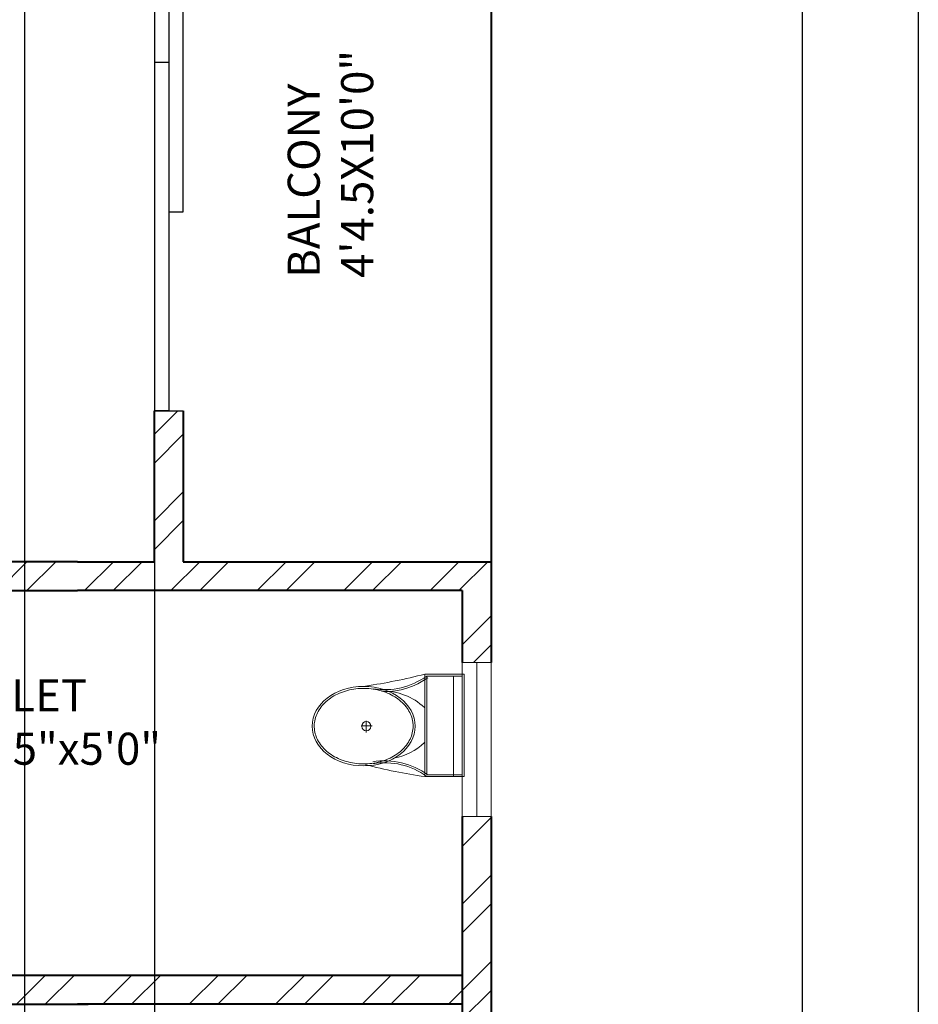
# Model space of a CAD drawing. Units: inches. Extents: x 1601 to 2297, y 1496 to 2631.
# Tile 26 of 57: x 2157 to 2297, y 1793 to 1946. Entities that reach past the tile are written whole.
import ezdxf

# ---------------------------------------------------------------- set-up
doc = ezdxf.new("R2010")
doc.units = ezdxf.units.IN
for name, color, linetype, lineweight in [('A-ANNO-DIMS', 2, 'Continuous', 18), ('A-ANNO-TTLB', 7, 'Continuous', 25), ('A-AREA-IDEN', 7, 'Continuous', 18), ('A-DOOR', 21, 'Continuous', 25), ('A-FLOR-FIXT', 9, 'Continuous', 20), ('A-GLAZ', 161, 'Continuous', 20), ('A-WALL', 7, 'Continuous', 40), ('A-WALL-PATT', 215, 'Continuous', 13)]:
    doc.layers.add(name, color=color, linetype=linetype, lineweight=lineweight)
doc.styles.get("Standard").update_dxf_attribs({"font": 'arial.ttf'})
doc.dimstyles.get("Standard").update_dxf_attribs({"dimtxt": 0.18, "dimasz": 0.18, "dimexe": 0.18, "dimexo": 0.0625, "dimgap": 0.09, "dimtad": 0, "dimtih": 1, "dimtoh": 1, "dimdec": 4, "dimzin": 0, "dimdsep": 46, "dimtxsty": 'Standard', "dimcen": 0.09, "dimadec": 0, "dimazin": 0, "dimtfac": 1, "dimtdec": 4, "dimtofl": 0, "dimtmove": 0, "dimatfit": 3, "dimfxl": 1, "dimtolj": 1, "dimtzin": 0, "dimarcsym": 0})

# ---------------------------------------------------------------- blocks, each defined once
blk = doc.blocks.new('A$C31115884')
for p, q in [((257.5, 466.4), (257.5, 523.2)), ((283.1, 497.7), (223.4, 497.7)), ((0, 200), (0, 0)), ((520, 200), (0, 200)), ((520, 0), (520, 200)), ((10, 190), (10, 10)), ((510, 190), (10, 190)), ((510, 10), (510, 190)), ((510, 54.5), (0, 54.5)), ((10, 10), (510, 10)), ((0, 0), (520, 0))]:
    blk.add_line(p, q)
blk.add_circle((255.6, 496.4), 23.6)
for centre, radius, start, end in [((2777.7, -204.6), 2807, 165.4549, 171.7133), ((3237, 905), 2807, 188.2867, 194.5451), ((-294.5, 403.3), 364.7, 324.2091, 9.3499), ((-294.5, 403.3), 374.7, 324.2091, 9.3499), ((805.8, 403.3), 364.7, 170.6501, 215.7909), ((139.5, 406.2), 293.5, 315.8436, 2.6563), ((805.8, 403.3), 374.7, 179.2036, 215.7909), ((383.6, 406.2), 293.5, 190.2774, 224.1564)]:
    blk.add_arc(centre, radius, start, end)
blk.add_ellipse((256.2, 509.9), major_axis=(0, -260.7), ratio=0.772727)
blk.add_open_spline([(256.2, 259.2), (263.1, 259.2), (270, 259.7), (287.8, 262.3), (298.7, 265.1), (319.9, 273.1), (330.2, 278.4), (350.1, 291.1), (359.7, 298.7), (377.7, 315.9), (386.2, 325.5), (401.7, 346.6), (408.8, 358.1), (421.3, 382.5), (426.8, 395.5), (435.9, 422.4), (439.5, 436.4), (444.8, 465.1), (446.5, 479.7), (447.9, 509.2), (447.6, 524), (445, 553.3), (442.7, 567.8), (436.3, 596), (432.1, 609.7), (421.9, 636), (416, 648.6), (402.5, 672.1), (395, 683), (378.6, 703), (369.8, 712.1), (351.1, 728), (341.3, 734.8), (320.9, 746.2), (310.4, 750.7), (288.9, 757.3), (278, 759.4), (256, 761), (245, 760.6), (223.1, 757.2), (212.3, 754.3), (191.1, 746.1), (180.8, 740.7), (160.9, 727.8), (151.4, 720.1), (133.5, 702.7), (125.1, 693), (109.6, 671.7), (102.6, 660.2), (90.2, 635.7), (84.9, 622.7), (76, 595.6), (72.4, 581.6), (67.2, 552.9), (65.6, 538.2), (64.4, 508.8), (64.8, 494), (67.5, 464.7), (69.9, 450.2), (76.6, 422), (80.8, 408.3), (91.1, 382.2), (97.2, 369.7), (110.8, 346.3), (118.4, 335.4), (134.8, 315.6), (143.7, 306.7), (162.4, 290.9), (172.3, 284.2), (192.8, 273), (203.3, 268.6), (224.8, 262.2), (235.8, 260.2), (249.9, 259.3), (253, 259.2), (256.2, 259.2)], degree=3, knots=[0, 0, 0, 0, 0.110105, 0.110105, 0.285049, 0.285049, 0.459994, 0.459994, 0.634938, 0.634938, 0.809882, 0.809882, 0.984827, 0.984827, 1.159771, 1.159771, 1.334715, 1.334715, 1.50966, 1.50966, 1.684604, 1.684604, 1.859549, 1.859549, 2.034493, 2.034493, 2.209437, 2.209437, 2.384382, 2.384382, 2.559326, 2.559326, 2.73427, 2.73427, 2.909215, 2.909215, 3.084159, 3.084159, 3.259103, 3.259103, 3.434048, 3.434048, 3.608992, 3.608992, 3.783936, 3.783936, 3.958881, 3.958881, 4.133825, 4.133825, 4.30877, 4.30877, 4.483714, 4.483714, 4.658658, 4.658658, 4.833603, 4.833603, 5.008547, 5.008547, 5.183491, 5.183491, 5.358436, 5.358436, 5.53338, 5.53338, 5.708324, 5.708324, 5.883269, 5.883269, 6.058213, 6.058213, 6.233158, 6.233158, 6.283185, 6.283185, 6.283185, 6.283185])
blk = doc.blocks.new('WIN-24IN-JAMB4P5')
for p, q in [((0, 24), (4.5, 24)), ((0, 24), (0, 0)), ((4.5, 24), (2.25, 24)), ((2.25, 24), (2.25, 0)), ((4.5, 24), (4.5, 0)), ((2.25, 0), (0, 0)), ((0, 0), (4.5, 0))]:
    blk.add_line(p, q)
blk = doc.blocks.new('*D29')
at = {"layer": 'A-ANNO-DIMS', "color": 0, "lineweight": -2, "transparency": 16777216}
for p, q in [((2230.6, 2532.33), (2279.27, 2532.33)), ((2279.09, 2532.15), (2279.09, 2084.01)), ((2279.09, 1635.51), (2279.09, 2083.64)), ((2230.6, 1635.33), (2279.27, 1635.33))]:
    blk.add_line(p, q, dxfattribs=at)
at = {"layer": 'A-ANNO-DIMS', "color": 0, "transparency": 16777216}
for points in [[(2279.06, 2532.15), (2279.12, 2532.15), (2279.09, 2532.33)], [(2279.06, 1635.51), (2279.12, 1635.51), (2279.09, 1635.33)]]:
    blk.add_solid(points, dxfattribs=at)
at = {"layer": 'Defpoints', "color": 0, "transparency": 16777216}
for p in [(2230.54, 2532.33), (2279.09, 2532.33), (2230.54, 1635.33)]:
    blk.add_point(p, dxfattribs=at)
at = {"layer": 'A-ANNO-DIMS', "color": 0, "transparency": 16777216, "insert": (2279.09, 2083.83), "char_height": 0.18, "attachment_point": 5}
blk.add_mtext('\\A1;897', dxfattribs=at)
blk = doc.blocks.new('*D38')
at = {"layer": 'A-ANNO-DIMS', "color": 0, "lineweight": -2, "transparency": 16777216}
for p, q in [((2178.04, 2085.26), (2178.04, 1513.75)), ((2157.8, 2066.51), (2157.8, 1513.75)), ((2157.98, 1513.93), (2167.52, 1513.93)), ((2177.86, 1513.93), (2168.31, 1513.93))]:
    blk.add_line(p, q, dxfattribs=at)
at = {"layer": 'A-ANNO-DIMS', "color": 0, "transparency": 16777216}
for points in [[(2157.98, 1513.96), (2157.98, 1513.9), (2157.8, 1513.93)], [(2177.86, 1513.96), (2177.86, 1513.9), (2178.04, 1513.93)]]:
    blk.add_solid(points, dxfattribs=at)
at = {"layer": 'Defpoints', "color": 0, "transparency": 16777216}
for p in [(2178.04, 2085.33), (2157.8, 2066.58), (2178.04, 1513.93)]:
    blk.add_point(p, dxfattribs=at)
at = {"layer": 'A-ANNO-DIMS', "color": 0, "transparency": 16777216, "insert": (2167.92, 1513.93), "char_height": 0.18, "attachment_point": 5}
blk.add_mtext('\\A1;20.24', dxfattribs=at)

msp = doc.modelspace()

# ---------------------------------------------------------------- hatches: boundary and pattern name
at = {"layer": 'A-WALL-PATT'}
h = msp.add_hatch(dxfattribs=at)
h.set_pattern_fill('ANSI32', color=256)
h.paths.add_polyline_path([(1842.0336, 2528.0767), (1842.0336, 2532.3254), (1686.0373, 2532.3254), (1686.0373, 2492.9493), (1695.0373, 2492.9493), (1695.0373, 2523.3254), (1827.0373, 2523.3254), (1827.0373, 2416.8254), (1834.6225, 2416.8254), (1834.6225, 2419.0754), (1834.6225, 2421.3254), (1831.5373, 2421.3254), (1831.5373, 2523.3254), (1842.0336, 2523.3254)])
h.paths.add_polyline_path([(1695.0373, 2432.9493), (1686.0373, 2432.9493), (1686.0373, 2325.989), (1695.0373, 2325.989), (1695.0373, 2347.8254), (1827.0373, 2347.8254), (1827.0373, 2287.8254), (1823.2991, 2287.8254), (1823.2991, 2283.3254), (1847.9422, 2283.3254), (1847.9422, 2285.5754), (1847.9422, 2287.8254), (1831.5373, 2287.8254), (1831.5373, 2347.8254), (1846.9946, 2347.8254), (1846.9946, 2350.0754), (1846.9946, 2352.3254), (1695.0373, 2352.3254)])
h.paths.add_polyline_path([(1807.1169, 1573.5395), (2055.0405, 1573.5395), (2055.0405, 1610.6322), (1807.1169, 1610.6322)], flags=9)
h.paths.add_polyline_path([(1841.1631, 1712.7967), (1870.3957, 1712.7967), (1870.3957, 1731.454), (1841.1631, 1731.454)], flags=9)
h.paths.add_polyline_path([(2144.3862, 1772.185), (2191.0233, 1772.185), (2191.0233, 1790.8423), (2144.3862, 1790.8423)], flags=9)
h.paths.add_polyline_path([(2143.0128, 1827.3312), (2177.9958, 1827.3312), (2177.9958, 1845.9886), (2143.0128, 1845.9886)], flags=9)
h.paths.add_polyline_path([(2041.2439, 1833.5691), (2070.8516, 1833.5691), (2070.8516, 1852.2264), (2041.2439, 1852.2264)], flags=9)
h.paths.add_polyline_path([(2097.2791, 1947.0598), (2134.2061, 1947.0598), (2134.2061, 1965.7171), (2097.2791, 1965.7171)], flags=9)
h.paths.add_polyline_path([(2214.995, 1904.3124), (2214.995, 1942.2899), (2196.3376, 1942.2899), (2196.3376, 1904.3124)], flags=9)
h.paths.add_polyline_path([(2186.6284, 2043.8031), (2219.7935, 2043.8031), (2219.7935, 2062.4605), (2186.6284, 2062.4605)], flags=9)
h.paths.add_polyline_path([(2064.0877, 2031.616), (2097.4949, 2031.616), (2097.4949, 2050.2734), (2064.0877, 2050.2734)], flags=9)
h.paths.add_polyline_path([(1973.1349, 1986.0688), (2008.4009, 1986.0688), (2008.4009, 2004.7261), (1973.1349, 2004.7261)], flags=9)
h.paths.add_polyline_path([(1976.3676, 2106.9635), (2005.7469, 2106.9635), (2005.7469, 2125.6209), (1976.3676, 2125.6209)], flags=9)
h.paths.add_polyline_path([(1991.7852, 2180.4863), (2027.0513, 2180.4863), (2027.0513, 2199.1437), (1991.7852, 2199.1437)], flags=9)
h.paths.add_polyline_path([(2106.1801, 2187.9359), (2152.2101, 2187.9359), (2152.2101, 2206.5932), (2106.1801, 2206.5932)], flags=9)
h.paths.add_polyline_path([(2148.6686, 2262.2542), (2182.318, 2262.2542), (2182.318, 2280.9115), (2148.6686, 2280.9115)], flags=9)
h.paths.add_polyline_path([(2041.6327, 2252.8147), (2071.2405, 2252.8147), (2071.2405, 2271.4721), (2041.6327, 2271.4721)], flags=9)
h.paths.add_polyline_path([(2063.9734, 2375.4265), (2100.9004, 2375.4265), (2100.9004, 2394.0839), (2063.9734, 2394.0839)], flags=9)
h.paths.add_polyline_path([(2216.4955, 2330.9748), (2216.4955, 2370.2654), (2197.8381, 2370.2654), (2197.8381, 2330.9748)], flags=9)
h.paths.add_polyline_path([(2179.1416, 2485.8687), (2212.3067, 2485.8687), (2212.3067, 2504.5261), (2179.1416, 2504.5261)], flags=9)
h.paths.add_polyline_path([(2078.7442, 2471.1516), (2112.1514, 2471.1516), (2112.1514, 2489.809), (2078.7442, 2489.809)], flags=9)
h.paths.add_polyline_path([(1915.9631, 2329.4668), (1952.8902, 2329.4668), (1952.8902, 2348.1241), (1915.9631, 2348.1241)], flags=9)
h.paths.add_polyline_path([(1904.3189, 2499.6709), (1940.4512, 2499.6709), (1940.4512, 2518.3282), (1904.3189, 2518.3282)], flags=9)
h.paths.add_polyline_path([(1892.3665, 2100.4595), (1925.6374, 2100.4595), (1925.6374, 2119.1169), (1892.3665, 2119.1169)], flags=9)
h.paths.add_polyline_path([(1909.2984, 1805.9631), (1946.2254, 1805.9631), (1946.2254, 1824.6205), (1909.2984, 1824.6205)], flags=9)
h.paths.add_polyline_path([(1934.6056, 1658.616), (1970.738, 1658.616), (1970.738, 1677.2733), (1934.6056, 1677.2733)], flags=9)
h.paths.add_polyline_path([(1711.2052, 1789.8902), (1750.0456, 1789.8902), (1750.0456, 1808.5476), (1711.2052, 1808.5476)], flags=9)
h.paths.add_polyline_path([(1742.7874, 1854.6743), (1771.9449, 1854.6743), (1771.9449, 1873.3317), (1742.7874, 1873.3317)], flags=9)
h.paths.add_polyline_path([(1807.3592, 1997.7912), (1850.1116, 1997.7912), (1850.1116, 2016.4486), (1807.3592, 2016.4486)], flags=9)
h.paths.add_polyline_path([(1717.4579, 2237.7844), (1760.2103, 2237.7844), (1760.2103, 2256.4417), (1717.4579, 2256.4417)], flags=9)
h.paths.add_polyline_path([(1780.9285, 2324.0623), (1810.086, 2324.0623), (1810.086, 2342.7197), (1780.9285, 2342.7197)], flags=25)
h.paths.add_polyline_path([(1837.696, 2449.2024), (1866.9286, 2449.2024), (1866.9286, 2467.8598), (1837.696, 2467.8598)], flags=9)
h.paths.add_polyline_path([(1712.7752, 2484.9404), (1751.6156, 2484.9404), (1751.6156, 2503.5977), (1712.7752, 2503.5977)], flags=25)
h = msp.add_hatch(dxfattribs=at)
h.set_pattern_fill('ANSI32', color=256)
h.paths.add_polyline_path([(1973.9371, 2211.3254), (1893.0373, 2211.3254), (1893.0373, 2287.8254), (1884.6167, 2287.8254), (1884.6167, 2285.5754), (1884.6167, 2283.3254), (1888.5373, 2283.3254), (1888.5373, 2145.3254), (1695.0373, 2145.3254), (1695.0373, 2173.8724), (1690.5373, 2173.8724), (1686.0373, 2173.8724), (1686.0373, 2136.3254), (1722.5687, 2136.3254), (1722.5687, 2117.4352), (1731.5687, 2117.4352), (1731.5687, 2136.3254), (1893.0373, 2136.3254), (1893.0373, 2202.3254), (1959.0373, 2202.3254), (1959.0373, 2182.1303), (1968.0373, 2182.1303), (1968.0373, 2202.3254), (1973.9371, 2202.3254)])
h.paths.add_polyline_path([(2094.0373, 2274.6364), (2096.4294, 2274.6364), (2096.4294, 2276.8864), (2096.4294, 2279.1364), (2094.0373, 2279.1364), (2094.0373, 2290.8254), (2094.0373, 2295.3254), (2089.5373, 2295.3254), (2089.5373, 2230.8254), (2035.5373, 2230.8254), (2035.5373, 2299.8254), (2031.0373, 2299.8254), (2031.0373, 2211.3254), (2023.0065, 2211.3254), (2023.0065, 2202.3254), (2031.0373, 2202.3254), (2031.0373, 2140.8254), (1968.0373, 2140.8254), (1968.0373, 2145.9106), (1963.5373, 2145.9106), (1959.0373, 2145.9106), (1959.0373, 2116.839), (1963.5373, 2116.839), (1968.0373, 2116.839), (1968.0373, 2131.8254), (2031.0373, 2131.8254), (2031.0373, 2094.3254), (2031.0373, 2085.3254), (2031.0373, 2056.8254), (1968.0373, 2056.8254), (1968.0373, 2070.4947), (1963.5373, 2070.4947), (1959.0373, 2070.4947), (1959.0373, 2040.3029), (1968.0373, 2040.3029), (1968.0373, 2047.8254), (2031.0373, 2047.8254), (2031.0373, 1983.3254), (2031.0373, 1978.8254), (2021.1979, 1978.8254), (2021.1979, 1974.3254), (2031.0373, 1974.3254), (2031.0373, 1954.3528), (2035.5373, 1954.3528), (2035.5373, 1974.3254), (2035.5373, 1981.8254), (2055.5513, 1981.8254), (2055.5513, 1986.3254), (2035.5373, 1986.3254), (2035.5373, 2047.8254), (2040.0373, 2047.8254), (2040.0373, 2085.3254), (2040.0373, 2094.3254), (2040.0373, 2140.8254), (2035.5373, 2140.8254), (2035.5373, 2226.3254), (2089.5373, 2226.3254), (2094.0373, 2226.3254)])
h.paths.add_polyline_path([(2226.0373, 2230.8254), (2134.5373, 2230.8254), (2134.5373, 2233.5437), (2130.0373, 2233.5437), (2130.0373, 2226.3254), (2134.5373, 2226.3254), (2226.0373, 2226.3254)])
h.paths.add_polyline_path([(1807.1169, 1573.5395), (2055.0405, 1573.5395), (2055.0405, 1610.6322), (1807.1169, 1610.6322)], flags=9)
h.paths.add_polyline_path([(1841.1631, 1712.7967), (1870.3957, 1712.7967), (1870.3957, 1731.454), (1841.1631, 1731.454)], flags=9)
h.paths.add_polyline_path([(2144.3862, 1772.185), (2191.0233, 1772.185), (2191.0233, 1790.8423), (2144.3862, 1790.8423)], flags=9)
h.paths.add_polyline_path([(2143.0128, 1827.3312), (2177.9958, 1827.3312), (2177.9958, 1845.9886), (2143.0128, 1845.9886)], flags=9)
h.paths.add_polyline_path([(2041.2439, 1833.5691), (2070.8516, 1833.5691), (2070.8516, 1852.2264), (2041.2439, 1852.2264)], flags=9)
h.paths.add_polyline_path([(2097.2791, 1947.0598), (2134.2061, 1947.0598), (2134.2061, 1965.7171), (2097.2791, 1965.7171)], flags=9)
h.paths.add_polyline_path([(2214.995, 1904.3124), (2214.995, 1942.2899), (2196.3376, 1942.2899), (2196.3376, 1904.3124)], flags=9)
h.paths.add_polyline_path([(2186.6284, 2043.8031), (2219.7935, 2043.8031), (2219.7935, 2062.4605), (2186.6284, 2062.4605)], flags=9)
h.paths.add_polyline_path([(2064.0877, 2031.616), (2097.4949, 2031.616), (2097.4949, 2050.2734), (2064.0877, 2050.2734)], flags=9)
h.paths.add_polyline_path([(1973.1349, 1986.0688), (2008.4009, 1986.0688), (2008.4009, 2004.7261), (1973.1349, 2004.7261)], flags=25)
h.paths.add_polyline_path([(1976.3676, 2106.9635), (2005.7469, 2106.9635), (2005.7469, 2125.6209), (1976.3676, 2125.6209)], flags=25)
h.paths.add_polyline_path([(1991.7852, 2180.4863), (2027.0513, 2180.4863), (2027.0513, 2199.1437), (1991.7852, 2199.1437)], flags=25)
h.paths.add_polyline_path([(2106.1801, 2187.9359), (2152.2101, 2187.9359), (2152.2101, 2206.5932), (2106.1801, 2206.5932)], flags=9)
h.paths.add_polyline_path([(2148.6686, 2262.2542), (2182.318, 2262.2542), (2182.318, 2280.9115), (2148.6686, 2280.9115)], flags=9)
h.paths.add_polyline_path([(2041.6327, 2252.8147), (2071.2405, 2252.8147), (2071.2405, 2271.4721), (2041.6327, 2271.4721)], flags=25)
h.paths.add_polyline_path([(2063.9734, 2375.4265), (2100.9004, 2375.4265), (2100.9004, 2394.0839), (2063.9734, 2394.0839)], flags=9)
h.paths.add_polyline_path([(2216.4955, 2330.9748), (2216.4955, 2370.2654), (2197.8381, 2370.2654), (2197.8381, 2330.9748)], flags=9)
h.paths.add_polyline_path([(2179.1416, 2485.8687), (2212.3067, 2485.8687), (2212.3067, 2504.5261), (2179.1416, 2504.5261)], flags=9)
h.paths.add_polyline_path([(2078.7442, 2471.1516), (2112.1514, 2471.1516), (2112.1514, 2489.809), (2078.7442, 2489.809)], flags=9)
h.paths.add_polyline_path([(1915.9631, 2329.4668), (1952.8902, 2329.4668), (1952.8902, 2348.1241), (1915.9631, 2348.1241)], flags=9)
h.paths.add_polyline_path([(1904.3189, 2499.6709), (1940.4512, 2499.6709), (1940.4512, 2518.3282), (1904.3189, 2518.3282)], flags=9)
h.paths.add_polyline_path([(1892.3665, 2100.4595), (1925.6374, 2100.4595), (1925.6374, 2119.1169), (1892.3665, 2119.1169)], flags=9)
h.paths.add_polyline_path([(1909.2984, 1805.9631), (1946.2254, 1805.9631), (1946.2254, 1824.6205), (1909.2984, 1824.6205)], flags=9)
h.paths.add_polyline_path([(1934.6056, 1658.616), (1970.738, 1658.616), (1970.738, 1677.2733), (1934.6056, 1677.2733)], flags=9)
h.paths.add_polyline_path([(1711.2052, 1789.8902), (1750.0456, 1789.8902), (1750.0456, 1808.5476), (1711.2052, 1808.5476)], flags=9)
h.paths.add_polyline_path([(1742.7874, 1854.6743), (1771.9449, 1854.6743), (1771.9449, 1873.3317), (1742.7874, 1873.3317)], flags=9)
h.paths.add_polyline_path([(1807.3592, 1997.7912), (1850.1116, 1997.7912), (1850.1116, 2016.4486), (1807.3592, 2016.4486)], flags=9)
h.paths.add_polyline_path([(1717.4579, 2237.7844), (1760.2103, 2237.7844), (1760.2103, 2256.4417), (1717.4579, 2256.4417)], flags=25)
h.paths.add_polyline_path([(1780.9285, 2324.0623), (1810.086, 2324.0623), (1810.086, 2342.7197), (1780.9285, 2342.7197)], flags=9)
h.paths.add_polyline_path([(1837.696, 2449.2024), (1866.9286, 2449.2024), (1866.9286, 2467.8598), (1837.696, 2467.8598)], flags=9)
h.paths.add_polyline_path([(1712.7752, 2484.9404), (1751.6156, 2484.9404), (1751.6156, 2503.5977), (1712.7752, 2503.5977)], flags=9)
h = msp.add_hatch(dxfattribs=at)
h.set_pattern_fill('ANSI32', color=256)
h.paths.add_polyline_path([(2230.5373, 1861.8254), (2182.5373, 1861.8254), (2182.5373, 1885.3637), (2178.0373, 1885.3637), (2178.0373, 1861.8254), (2166.0373, 1861.8254), (2134.5373, 1861.8254), (2130.0373, 1861.8254), (2130.0373, 1841.4682), (2126.8833, 1841.4682), (2126.8833, 1836.9682), (2130.0373, 1836.9682), (2130.0373, 1822.7302), (2134.5373, 1822.7302), (2134.5373, 1857.3254), (2166.0373, 1857.3254), (2226.0373, 1857.3254), (2226.0373, 1846.1155), (2230.5373, 1846.1155)])
h.paths.add_polyline_path([(2226.0373, 1797.3254), (2134.5373, 1797.3254), (2134.5373, 1800.6636), (2132.2873, 1800.6636), (2130.0373, 1800.6636), (2130.0373, 1797.3254), (2130.0373, 1792.8254), (2167.7264, 1792.8254), (2226.0373, 1792.8254)])
h.paths.add_polyline_path([(2230.5373, 1822.1155), (2226.0373, 1822.1155), (2226.0373, 1760.8563), (2230.5373, 1760.8563)])
h.paths.add_polyline_path([(2230.5373, 1700.8563), (2226.0373, 1700.8563), (2226.0373, 1644.3254), (2140.2517, 1644.3254), (2140.2517, 1635.3254), (2230.5373, 1635.3254)])
h.paths.add_polyline_path([(2080.2517, 1639.8254), (2080.2517, 1644.3254), (2035.5373, 1644.3254), (2035.5373, 1792.8254), (2094.0373, 1792.8254), (2094.0373, 1797.3254), (2094.0373, 1836.9682), (2097.1057, 1836.9682), (2097.1057, 1839.2182), (2097.1057, 1841.4682), (2094.0373, 1841.4682), (2094.0373, 1862.2276), (2089.5373, 1862.2276), (2089.5373, 1797.3254), (2035.5373, 1797.3254), (2035.5373, 1857.3254), (2035.5373, 1885.0916), (2031.0373, 1885.0916), (2031.0373, 1710.3254), (2012.329, 1710.3254), (2012.329, 1701.3254), (2031.0373, 1701.3254), (2031.0373, 1644.3254), (2031.0373, 1635.3254), (2080.2517, 1635.3254)])
h.paths.add_polyline_path([(1836.0373, 1653.2033), (1842.6171, 1653.2033), (1842.6171, 1657.7033), (1842.6171, 1662.2033), (1831.5373, 1662.2033), (1831.5373, 1764.2033), (1835.3881, 1764.2033), (1835.3881, 1766.4533), (1835.3881, 1768.7033), (1831.5373, 1768.7033), (1827.0373, 1768.7033), (1827.0373, 1662.2033), (1827.0373, 1635.3254), (1836.0373, 1635.3254)])
h.paths.add_polyline_path([(1893.0373, 1701.3254), (1907.193, 1701.3254), (1907.193, 1705.8254), (1907.193, 1710.3254), (1893.0373, 1710.3254), (1893.0373, 1819.8254), (1882.6444, 1819.8254), (1882.6444, 1817.5754), (1882.6444, 1815.3254), (1888.5373, 1815.3254), (1888.5373, 1662.2033), (1884.0373, 1662.2033), (1866.6171, 1662.2033), (1866.6171, 1653.2033), (1882.391, 1653.2033), (1884.0373, 1653.2033), (1884.0373, 1635.3254), (1893.0373, 1635.3254)])
h.paths.add_polyline_path([(1739.3335, 1639.8254), (1739.3335, 1644.3254), (1695.0373, 1644.3254), (1695.0373, 1702.0135), (1690.5373, 1702.0135), (1686.0373, 1702.0135), (1686.0373, 1635.3254), (1739.3335, 1635.3254)])
h.paths.add_polyline_path([(1827.0373, 1644.3254), (1799.3335, 1644.3254), (1799.3335, 1635.3254), (1827.0373, 1635.3254)])
h.paths.add_polyline_path([(1695.0373, 1815.3254), (1849.2759, 1815.3254), (1849.2759, 1819.8254), (1807.5373, 1819.8254), (1807.5373, 1879.8254), (1851.1533, 1879.8254), (1851.1533, 1882.0754), (1851.1533, 1884.3254), (1799.3405, 1884.3254), (1799.3405, 1882.0754), (1799.3405, 1879.8254), (1803.0373, 1879.8254), (1803.0373, 1819.8254), (1695.0373, 1819.8254), (1695.0373, 1835.0458), (1690.5373, 1835.0458), (1686.0373, 1835.0458), (1686.0373, 1766.1753), (1695.0373, 1766.1753)])
h.paths.add_polyline_path([(1775.8157, 1884.3254), (1695.0373, 1884.3254), (1695.0373, 1912.9526), (1690.5373, 1912.9526), (1686.0373, 1912.9526), (1686.0373, 1859.0458), (1695.0373, 1859.0458), (1695.0373, 1879.8254), (1775.8157, 1879.8254)])
h.paths.add_polyline_path([(1893.0373, 2031.3254), (1731.5687, 2031.3254), (1731.5687, 2057.4352), (1722.5687, 2057.4352), (1722.5687, 2031.3254), (1686.0373, 2031.3254), (1686.0373, 1972.9526), (1695.0373, 1972.9526), (1695.0373, 2022.3254), (1888.5373, 2022.3254), (1888.5373, 1884.3254), (1883.4996, 1884.3254), (1883.4996, 1879.8254), (1893.0373, 1879.8254), (1893.0373, 1974.3254), (1976.6199, 1974.3254), (1976.6199, 1978.8254), (1968.0373, 1978.8254), (1968.0373, 1983.3254), (1968.0373, 2008.4756), (1963.5373, 2008.4756), (1959.0373, 2008.4756), (1959.0373, 1983.3254), (1893.0373, 1983.3254)])
h.paths.add_polyline_path([(2230.5373, 2140.4745), (2226.0373, 2140.4745), (2226.0373, 2094.3254), (2040.0373, 2094.3254), (2040.0373, 2085.3254), (2178.0373, 2085.3254), (2178.0373, 2065.6965), (2182.5373, 2065.6965), (2182.5373, 2085.3254), (2226.0373, 2085.3254), (2226.0373, 1986.3254), (2211.2679, 1986.3254), (2211.2679, 1981.8254), (2230.5373, 1981.8254)])
h.paths.add_polyline_path([(2187.6292, 1986.3254), (2182.5373, 1986.3254), (2182.5373, 2029.6965), (2178.0373, 2029.6965), (2178.0373, 1986.3254), (2099.05, 1986.3254), (2099.05, 1981.8254), (2178.0373, 1981.8254), (2178.0373, 1969.3637), (2182.5373, 1969.3637), (2182.5373, 1981.8254), (2187.6292, 1981.8254), (2187.6292, 1984.0754)])
h.paths.add_polyline_path([(1807.1169, 1573.5395), (2055.0405, 1573.5395), (2055.0405, 1610.6322), (1807.1169, 1610.6322)], flags=9)
h.paths.add_polyline_path([(1841.1631, 1712.7967), (1870.3957, 1712.7967), (1870.3957, 1731.454), (1841.1631, 1731.454)], flags=9)
h.paths.add_polyline_path([(2144.3862, 1772.185), (2191.0233, 1772.185), (2191.0233, 1790.8423), (2144.3862, 1790.8423)], flags=9)
h.paths.add_polyline_path([(2143.0128, 1827.3312), (2177.9958, 1827.3312), (2177.9958, 1845.9886), (2143.0128, 1845.9886)], flags=25)
h.paths.add_polyline_path([(2041.2439, 1833.5691), (2070.8516, 1833.5691), (2070.8516, 1852.2264), (2041.2439, 1852.2264)], flags=25)
h.paths.add_polyline_path([(2097.2791, 1947.0598), (2134.2061, 1947.0598), (2134.2061, 1965.7171), (2097.2791, 1965.7171)], flags=9)
h.paths.add_polyline_path([(2214.995, 1904.3124), (2214.995, 1942.2899), (2196.3376, 1942.2899), (2196.3376, 1904.3124)], flags=9)
h.paths.add_polyline_path([(2186.6284, 2043.8031), (2219.7935, 2043.8031), (2219.7935, 2062.4605), (2186.6284, 2062.4605)], flags=25)
h.paths.add_polyline_path([(2064.0877, 2031.616), (2097.4949, 2031.616), (2097.4949, 2050.2734), (2064.0877, 2050.2734)], flags=25)
h.paths.add_polyline_path([(1973.1349, 1986.0688), (2008.4009, 1986.0688), (2008.4009, 2004.7261), (1973.1349, 2004.7261)], flags=9)
h.paths.add_polyline_path([(1976.3676, 2106.9635), (2005.7469, 2106.9635), (2005.7469, 2125.6209), (1976.3676, 2125.6209)], flags=9)
h.paths.add_polyline_path([(1991.7852, 2180.4863), (2027.0513, 2180.4863), (2027.0513, 2199.1437), (1991.7852, 2199.1437)], flags=9)
h.paths.add_polyline_path([(2106.1801, 2187.9359), (2152.2101, 2187.9359), (2152.2101, 2206.5932), (2106.1801, 2206.5932)], flags=9)
h.paths.add_polyline_path([(2148.6686, 2262.2542), (2182.318, 2262.2542), (2182.318, 2280.9115), (2148.6686, 2280.9115)], flags=9)
h.paths.add_polyline_path([(2041.6327, 2252.8147), (2071.2405, 2252.8147), (2071.2405, 2271.4721), (2041.6327, 2271.4721)], flags=9)
h.paths.add_polyline_path([(2063.9734, 2375.4265), (2100.9004, 2375.4265), (2100.9004, 2394.0839), (2063.9734, 2394.0839)], flags=9)
h.paths.add_polyline_path([(2216.4955, 2330.9748), (2216.4955, 2370.2654), (2197.8381, 2370.2654), (2197.8381, 2330.9748)], flags=9)
h.paths.add_polyline_path([(2179.1416, 2485.8687), (2212.3067, 2485.8687), (2212.3067, 2504.5261), (2179.1416, 2504.5261)], flags=9)
h.paths.add_polyline_path([(2078.7442, 2471.1516), (2112.1514, 2471.1516), (2112.1514, 2489.809), (2078.7442, 2489.809)], flags=9)
h.paths.add_polyline_path([(1915.9631, 2329.4668), (1952.8902, 2329.4668), (1952.8902, 2348.1241), (1915.9631, 2348.1241)], flags=9)
h.paths.add_polyline_path([(1904.3189, 2499.6709), (1940.4512, 2499.6709), (1940.4512, 2518.3282), (1904.3189, 2518.3282)], flags=9)
h.paths.add_polyline_path([(1892.3665, 2100.4595), (1925.6374, 2100.4595), (1925.6374, 2119.1169), (1892.3665, 2119.1169)], flags=9)
h.paths.add_polyline_path([(1909.2984, 1805.9631), (1946.2254, 1805.9631), (1946.2254, 1824.6205), (1909.2984, 1824.6205)], flags=9)
h.paths.add_polyline_path([(1934.6056, 1658.616), (1970.738, 1658.616), (1970.738, 1677.2733), (1934.6056, 1677.2733)], flags=9)
h.paths.add_polyline_path([(1711.2052, 1789.8902), (1750.0456, 1789.8902), (1750.0456, 1808.5476), (1711.2052, 1808.5476)], flags=25)
h.paths.add_polyline_path([(1742.7874, 1854.6743), (1771.9449, 1854.6743), (1771.9449, 1873.3317), (1742.7874, 1873.3317)], flags=25)
h.paths.add_polyline_path([(1807.3592, 1997.7912), (1850.1116, 1997.7912), (1850.1116, 2016.4486), (1807.3592, 2016.4486)], flags=25)
h.paths.add_polyline_path([(1717.4579, 2237.7844), (1760.2103, 2237.7844), (1760.2103, 2256.4417), (1717.4579, 2256.4417)], flags=9)
h.paths.add_polyline_path([(1780.9285, 2324.0623), (1810.086, 2324.0623), (1810.086, 2342.7197), (1780.9285, 2342.7197)], flags=9)
h.paths.add_polyline_path([(1837.696, 2449.2024), (1866.9286, 2449.2024), (1866.9286, 2467.8598), (1837.696, 2467.8598)], flags=9)
h.paths.add_polyline_path([(1712.7752, 2484.9404), (1751.6156, 2484.9404), (1751.6156, 2503.5977), (1712.7752, 2503.5977)], flags=9)

# ---------------------------------------------------------------- linework, layer by layer
at = {"layer": 'A-ANNO-TTLB'}
msp.add_lwpolyline([(1600.5933, 2631.1477), (2297.129, 2631.1477), (2297.129, 1496.1026), (1600.5933, 1496.1026)], close=True, dxfattribs=at)
at = {"layer": 'A-DOOR'}
for p, q in [((2180.2873, 1969.3637), (2180.2873, 1885.3637)), ((2182.5373, 1916.3821), (2182.5373, 1969.3637)), ((2178.0373, 1939.7045), (2178.0373, 1885.3637)), ((2178.0373, 1939.7045), (2180.2873, 1939.7045)), ((2180.2873, 1916.3821), (2182.5373, 1916.3821)), ((2180.2873, 1885.3637), (2178.0373, 1885.3637)), ((2178.0373, 1885.3637), (2182.5373, 1885.3637))]:
    msp.add_line(p, q, dxfattribs=at)
at = {"layer": 'A-WALL'}
for p, q in [((2230.5373, 2140.4745), (2230.5373, 1846.1155)), ((2178.0373, 1861.8254), (2178.0373, 1885.3637)), ((2182.5373, 1885.3637), (2182.5373, 1861.8254)), ((2166.0373, 1861.8254), (2134.5373, 1861.8254)), ((2166.0373, 1861.8254), (2178.0373, 1861.8254)), ((2182.5373, 1861.8254), (2230.5373, 1861.8254)), ((2134.5373, 1857.3254), (2166.0373, 1857.3254)), ((2226.0373, 1857.3254), (2166.0373, 1857.3254)), ((2226.0373, 1857.3254), (2226.0373, 1846.1155)), ((2226.0373, 1857.3254), (2226.0373, 1846.1155)), ((2226.0373, 1822.1155), (2226.0373, 1797.3254)), ((2226.0373, 1822.1155), (2226.0373, 1760.8563)), ((2230.5373, 1822.1155), (2230.5373, 1760.8563)), ((2226.0373, 1797.3254), (2134.5373, 1797.3254)), ((2226.0373, 1797.3254), (2166.0373, 1797.3254)), ((2130.0373, 1792.8254), (2167.7264, 1792.8254)), ((2226.0373, 1792.8254), (2166.0373, 1792.8254))]:
    msp.add_line(p, q, dxfattribs=at)

# ---------------------------------------------------------------- block references
at = {"layer": 'A-FLOR-FIXT', "xscale": 0.0307498789965588, "yscale": 0.0307498789965588, "zscale": 0.0307498789965588, "rotation": 89.99999999999999}
msp.add_blockref('A$C31115884', (2226.3448, 1828.3162), dxfattribs=at)
at = {"layer": 'A-GLAZ'}
msp.add_blockref('WIN-24IN-JAMB4P5', (2226.037, 1822.1151), dxfattribs=at)

# ---------------------------------------------------------------- texts
at = {"layer": 'A-AREA-IDEN', "insert": (2198.8223, 1906.074), "char_height": 5, "attachment_point": 1, "rotation": 90}
msp.add_mtext_dynamic_manual_height_columns('BALCONY\\P4\'4.5X10\'0"', width=33.074822, gutter_width=12.5, heights=[0], dxfattribs=at)
at = {"layer": 'A-AREA-IDEN', "insert": (2144.5937, 1843.5039), "char_height": 5, "attachment_point": 1}
msp.add_mtext_dynamic_manual_height_columns('TOILET\\P7\'7.5"x5\'0"', width=77.548495, gutter_width=12.5, heights=[0], dxfattribs=at)

# ---------------------------------------------------------------- dimensions: what is measured, and where the dimension line sits
at = {"layer": 'A-ANNO-DIMS'}
dim = msp.add_linear_dim(base=(2279.0873, 2532.3254), p1=(2230.5373, 1635.3254), p2=(2230.5373, 2532.3254), angle=90, dimstyle='Standard', override={"dimdec": 0, "dimlfac": 1, "dimrnd": 0, "dimzin": 0, "dimdsep": 46, "dimlunit": 2}, dxfattribs=at)
dim.commit()
dim.dimension.update_dxf_attribs({"geometry": '*D29', "text_midpoint": (2279.0873, 2083.8254)})
dim = msp.add_linear_dim(base=(2178.0373, 1513.9279), p1=(2157.799, 2066.5754), p2=(2178.0373, 2085.3254), dimstyle='Standard', override={"dimdec": 2, "dimlfac": 1, "dimrnd": 0, "dimzin": 0, "dimdsep": 46, "dimlunit": 2}, dxfattribs=at)
dim.commit()
dim.dimension.update_dxf_attribs({"geometry": '*D38', "text_midpoint": (2167.9181, 1513.9279)})

doc.saveas('drawing.dxf')
